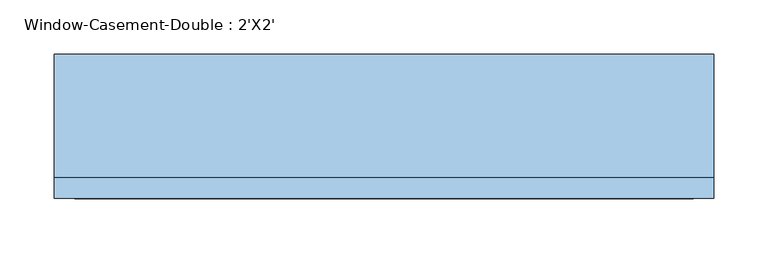
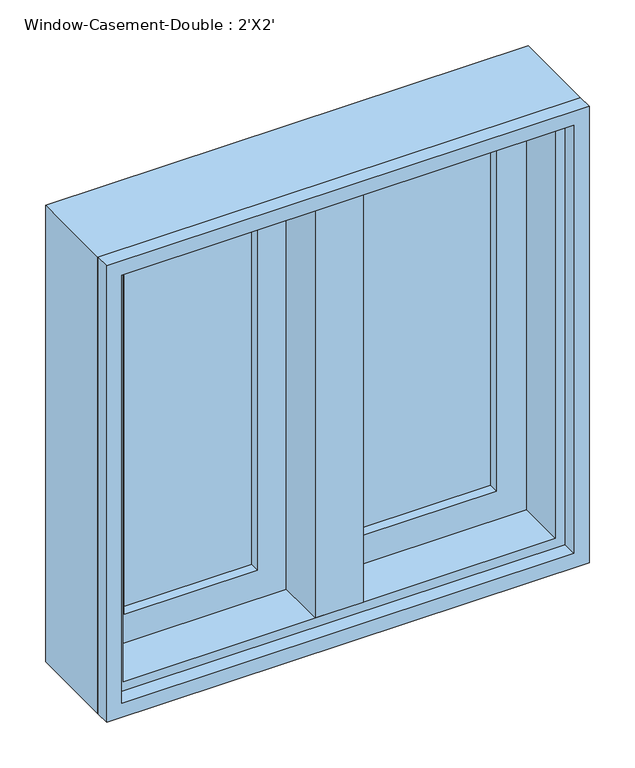
"""IFC4 building model written with IfcOpenShell, lengths in millimetres: window geometry, Window-Casement-Double : 2'X2'."""

from ifc_helpers import new_model, si_unit, frame, origin, place, context, project, spatial, polyline, outline, extrude, faceted_brep, source, transform, mapped, element, save


def window_casement_double_2_x2_e4709907(model_context):
    return source(origin(), model_context, "Body", "SolidModel", [
        faceted_brep([(9.525, 76.2, 1511.3), (-9.525, 76.2, 1511.3), (-9.525, 25.4, 1511.3), (9.525, 25.4, 1511.3), (9.525, 76.2, 927.1), (9.525, 25.4, 927.1), (-9.525, 25.4, 927.1), (-9.525, 76.2, 927.1), (-9.525, 25.4, 946.15), (-9.525, 25.4, 1492.25), (-30.1625, 25.4, 946.15), (-30.1625, 25.4, 1492.25), (-30.1625, -38.1, 946.15), (-30.1625, -38.1, 1492.25), (30.1625, -38.1, 946.15), (30.1625, -38.1, 1492.25), (30.1625, 25.4, 946.15), (30.1625, 25.4, 1492.25), (9.525, 25.4, 946.15), (9.525, 25.4, 1492.25)], [[[0, 1, 2, 3]], [[4, 5, 6, 7]], [[1, 0, 4, 7]], [[2, 1, 7, 6, 8, 9]], [[9, 8, 10, 11]], [[11, 10, 12, 13]], [[13, 12, 14, 15]], [[15, 14, 16, 17]], [[17, 16, 18, 19]], [[0, 3, 19, 18, 5, 4]], [[18, 8, 6, 5]], [[9, 19, 3, 2]], [[8, 18, 16, 14, 12, 10]], [[19, 9, 11, 13, 15, 17]]]),
        extrude(outline(polyline([(-66.675, 57.15), (-66.675, 50.8), (-234.95, 50.8), (-234.95, 57.15), (-66.675, 57.15)])), frame((0.0, 0.0, 984.25), z_axis=(0.0, 0.0, 1.0), x_axis=(1.0, 0.0, 0.0)), (0.0, 0.0, 1.0), 469.9),
        extrude(outline(polyline([(-234.95, 38.1), (-234.95, 44.45), (-66.675, 44.45), (-66.675, 38.1), (-234.95, 38.1)])), frame((0.0, 0.0, 984.25), z_axis=(0.0, 0.0, 1.0), x_axis=(1.0, 0.0, 0.0)), (0.0, 0.0, 1.0), 469.9),
        extrude(outline(polyline([(234.95, 57.15), (234.95, 50.8), (66.675, 50.8), (66.675, 57.15), (234.95, 57.15)])), frame((0.0, 0.0, 984.25), z_axis=(0.0, 0.0, 1.0), x_axis=(1.0, 0.0, 0.0)), (0.0, 0.0, 1.0), 469.9),
        extrude(outline(polyline([(66.675, 38.1), (66.675, 44.45), (234.95, 44.45), (234.95, 38.1), (66.675, 38.1)])), frame((0.0, 0.0, 984.25), z_axis=(0.0, 0.0, 1.0), x_axis=(1.0, 0.0, 0.0)), (0.0, 0.0, 1.0), 469.9),
        extrude(outline(polyline([(1511.3, -292.1), (927.1, -292.1), (927.1, -9.525), (1511.3, -9.525), (1511.3, -292.1)]), holes=[polyline([(1454.15, -66.675), (984.25, -66.675), (984.25, -234.95), (1454.15, -234.95), (1454.15, -66.675)])]), frame((0.0, 25.4, 0.0), z_axis=(0.0, 1.0, 0.0), x_axis=(0.0, 0.0, 1.0)), (0.0, 0.0, 1.0), 44.45),
        extrude(outline(polyline([(927.1, 292.1), (1511.3, 292.1), (1511.3, 9.525), (927.1, 9.525), (927.1, 292.1)]), holes=[polyline([(984.25, 66.675), (1454.15, 66.675), (1454.15, 234.95), (984.25, 234.95), (984.25, 66.675)])]), frame((0.0, 25.4, 0.0), z_axis=(0.0, 1.0, 0.0), x_axis=(0.0, 0.0, 1.0)), (0.0, 0.0, 1.0), 44.45),
        extrude(outline(polyline([(1524.0, -304.8), (914.4, -304.8), (914.4, 304.8), (1524.0, 304.8), (1524.0, -304.8)]), holes=[polyline([(1504.95, 285.75), (933.45, 285.75), (933.45, -285.75), (1504.95, -285.75), (1504.95, 285.75)])]), frame((0.0, -57.15, 0.0), z_axis=(0.0, 1.0, 0.0), x_axis=(0.0, 0.0, 1.0)), (0.0, 0.0, 1.0), 19.05),
        faceted_brep([(273.05, 25.4, 1492.25), (273.05, -38.1, 1492.25), (-273.05, -38.1, 1492.25), (-273.05, 25.4, 1492.25), (292.1, 76.2, 1511.3), (292.1, 25.4, 1511.3), (-292.1, 25.4, 1511.3), (-292.1, 76.2, 1511.3), (304.8, -38.1, 1524.0), (304.8, 76.2, 1524.0), (-304.8, 76.2, 1524.0), (-304.8, -38.1, 1524.0), (-273.05, -38.1, 946.15), (-273.05, 25.4, 946.15), (-292.1, 25.4, 927.1), (-292.1, 76.2, 927.1), (-304.8, 76.2, 914.4), (-304.8, -38.1, 914.4), (273.05, -38.1, 946.15), (273.05, 25.4, 946.15), (292.1, 25.4, 927.1), (292.1, 76.2, 927.1), (304.8, 76.2, 914.4), (304.8, -38.1, 914.4)], [[[0, 1, 2, 3]], [[4, 5, 6, 7]], [[8, 9, 10, 11]], [[3, 2, 12, 13]], [[7, 6, 14, 15]], [[11, 10, 16, 17]], [[13, 12, 18, 19]], [[15, 14, 20, 21]], [[17, 16, 22, 23]], [[11, 17, 23, 8], [1, 18, 12, 2]], [[19, 18, 1, 0]], [[5, 20, 14, 6], [3, 13, 19, 0]], [[21, 20, 5, 4]], [[23, 22, 9, 8]], [[9, 22, 16, 10], [7, 15, 21, 4]]]),
    ])


if __name__ == "__main__":
    model = new_model("IFC4")
    model_context = context("Model", 3, world=origin())
    ifc_project = project(units=[si_unit("LENGTHUNIT", "METRE", prefix="MILLI")], contexts=[model_context])
    site = spatial("IfcSite", under=ifc_project)
    building = spatial("IfcBuilding", under=site)
    placement = place(None, origin())
    window_casement_double_2_x2_shape = window_casement_double_2_x2_e4709907(model_context)
    element("IfcWindow", 1, ObjectType="Window-Casement-Double : 2'X2'", at=placement, inside=building, context=model_context, shape_type="MappedRepresentation", body=[
        mapped(window_casement_double_2_x2_shape, transform((0.0, 0.0, 0.0), x_axis=(1.0, 0.0, 0.0), y_axis=(0.0, 1.0, 0.0), z_axis=(0.0, 0.0, 1.0))),
    ])
    save(model, "model.ifc")

# Revit data of these elements
# Type "Window-Casement-Double : 2'X2'"
#   Type Mark = "20"
#   Fire Rating = "0.5h"
#   Assembly Code = "B2020100"
#   Analytic Construction = "Double glazing - domestic"
#   Frame Extension [instance default] = 0' - 0 1/4"
#   Window Inset [instance default] = 0' - 0"
#   Wall Thickness [instance default] = 0' - 6"
#   Interior Wall Closure [instance default] = 0' - 2 1/4"
#   Half Width = 1' - 0"
#   Visual Light Transmittance = 0.81
#   Thermal Resistance (R) = 1.8146 (h·ft²·°F)/BTU
#   Solar Heat Gain Coefficient = 0.76
#   Rough Width = 2' - 0 1/2"
#   Rough Height = 2' - 0 1/2"
#   Height = 2' - 0"
#   Heat Transfer Coefficient (U) = 0.5511 BTU/(h·ft²·°F)
#   Exterior Wall Closure [instance default] = 0' - 1 1/4"
#   Extension Jamb [instance default] = 0' - 2 1/4"
#   Default Sill Height = 3' - 0"
#   Width = 2' - 0"
#   Muntin Visibility = yes
#   Interior Trim Visibility [instance default] = yes
#   Exterior Trim Visibility [instance default] = yes
#   Extension Jamb Visibility [instance default] = yes
#   Interior Trim Material = Wood - Stained
#   Muntin Pattern = Muntin Pattern_2x2 : Muntin Pattern_2x2
#   Interior Trim = Trim-Window-Interior-Flat : Picture Frame
#   Interior Frame Material = Wood - Stained
#   Glass Panel Material = Glass
#   Exterior Trim Material = Clad - White
#   Exterior Trim = Trim-Window-Exterior-Flat : with Sill
#   Exterior Frame Material = Clad - White
#   Wall Closure = (empty or 0)
# Element 1 (IfcWindow, "Window-Casement-Double : 2'X2'")
#   Wall Thickness = 0' - 4 1/2"
#   Extension Jamb = 0' - 0 3/4"
#   Materials on its faces: "Wood - Stained", "Glass", "Clad - White"
# Materials
#   "Wood - Stained": class "Wood", colour RGB 224 178 126, transparency 0, Cost = 0
#   "Glass": class "Glass", colour RGB 0 128 192, transparency 0.75, Description = "Soda Lime Glass", Cost = 0
#   "Clad - White": class "Wood", colour RGB 242 242 238, transparency 0, Cost = 0
